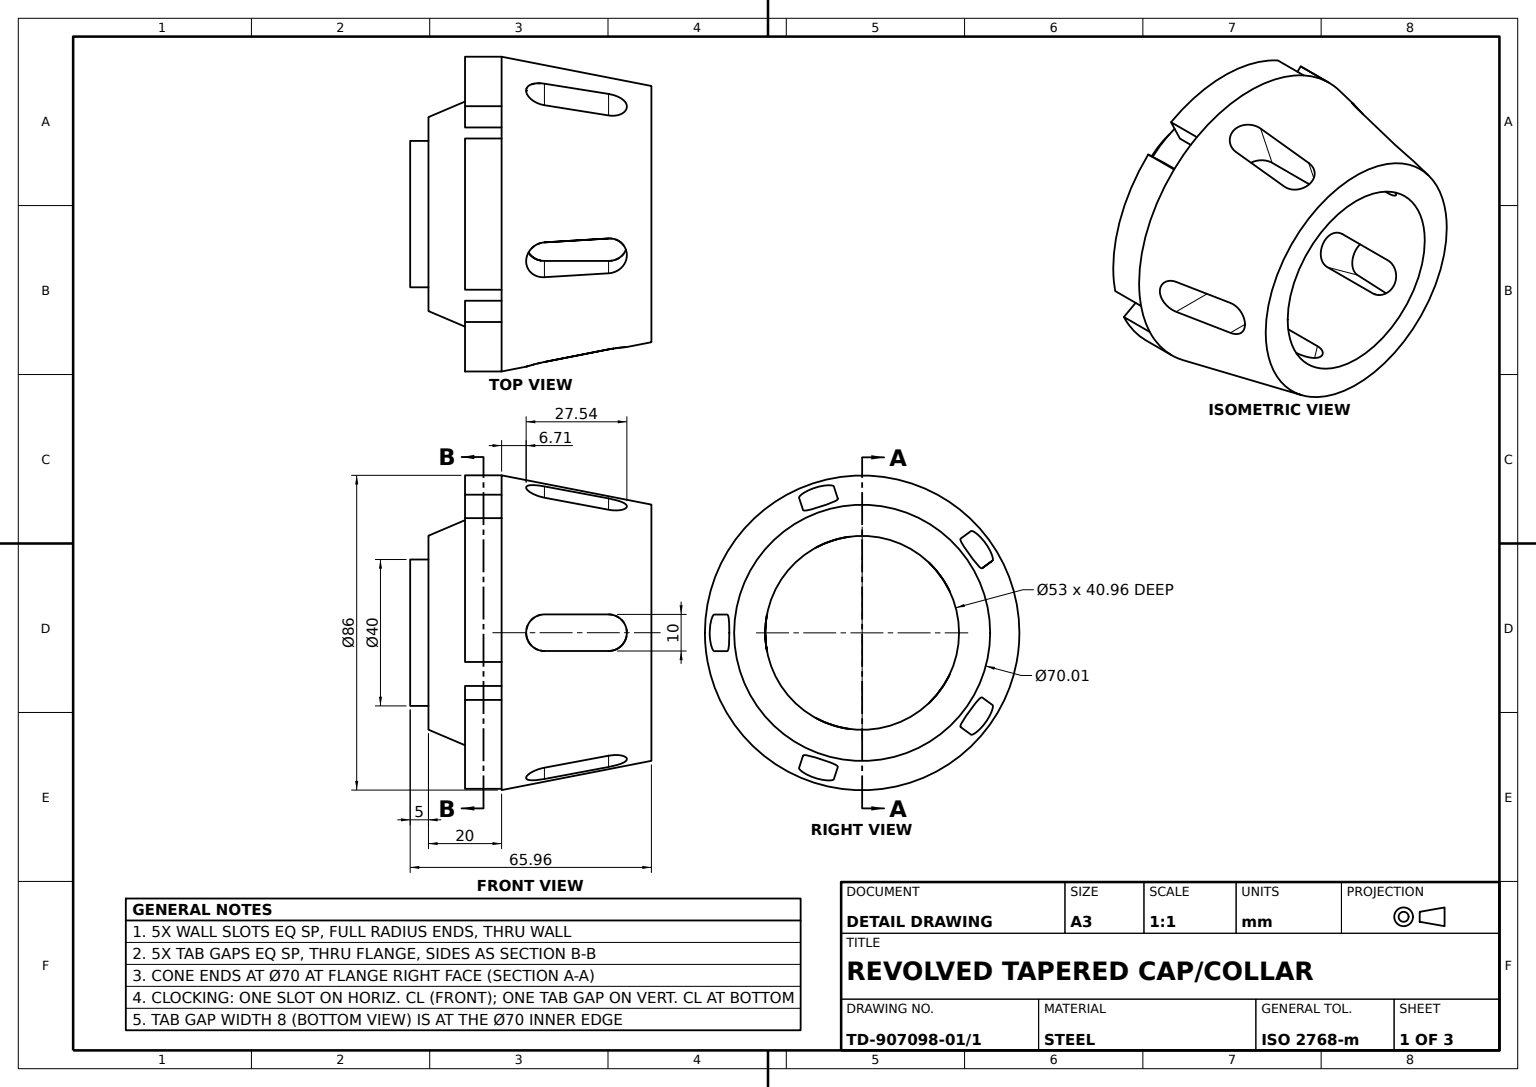
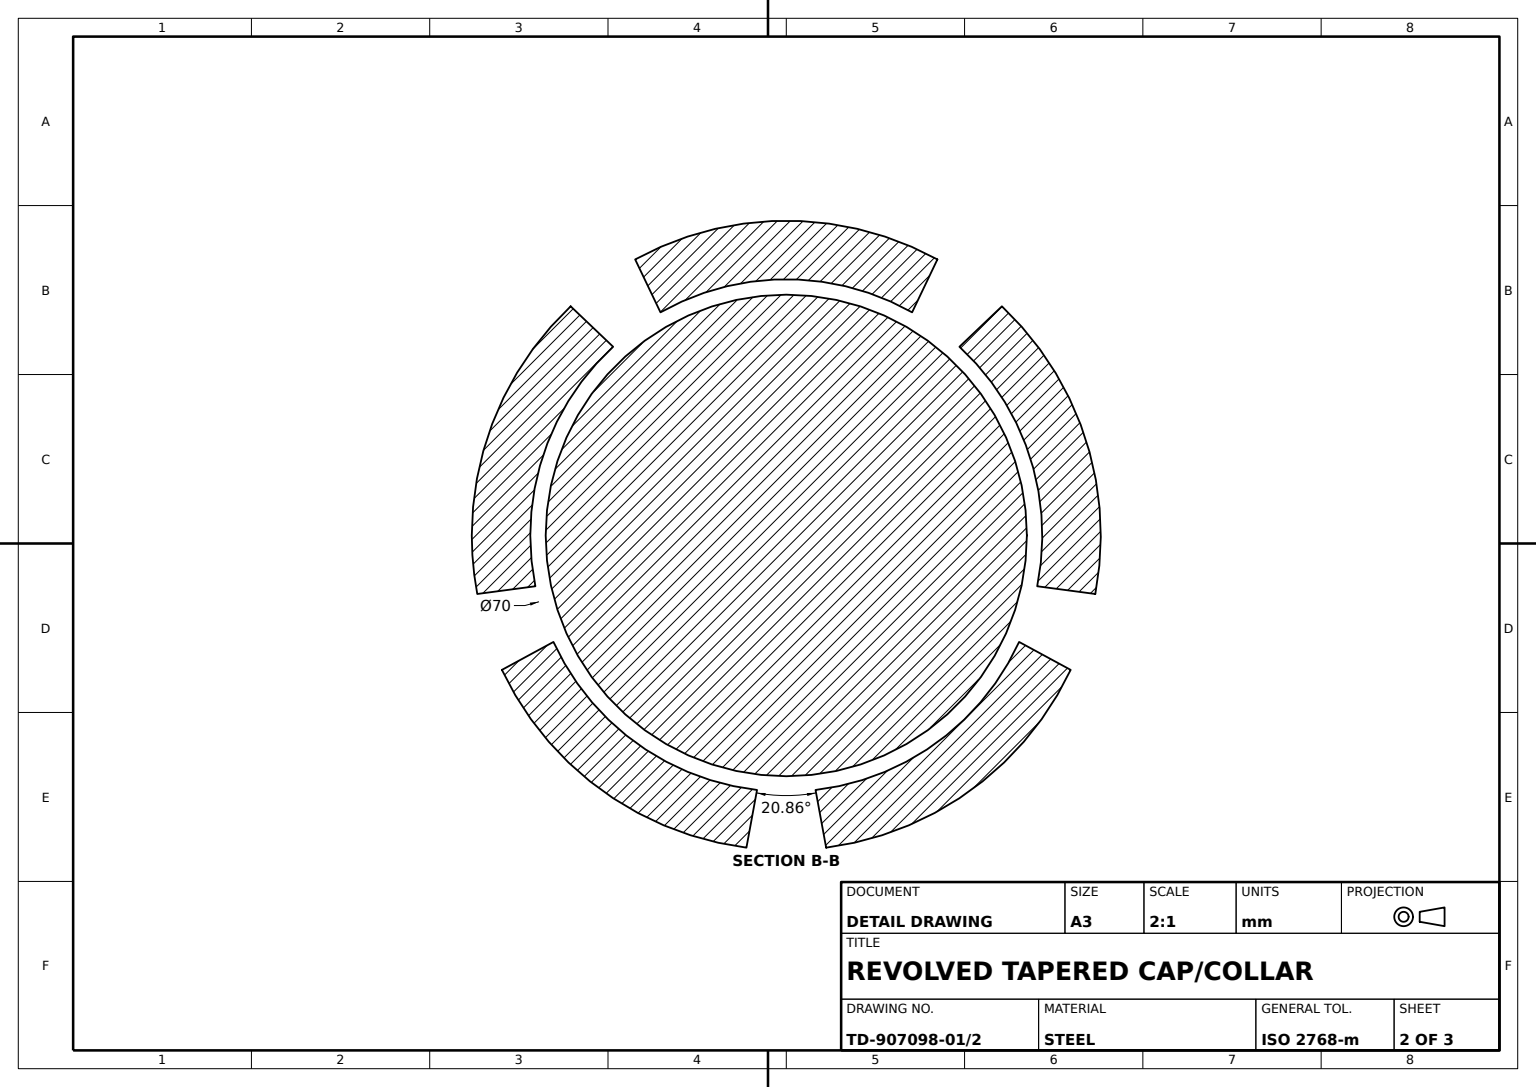
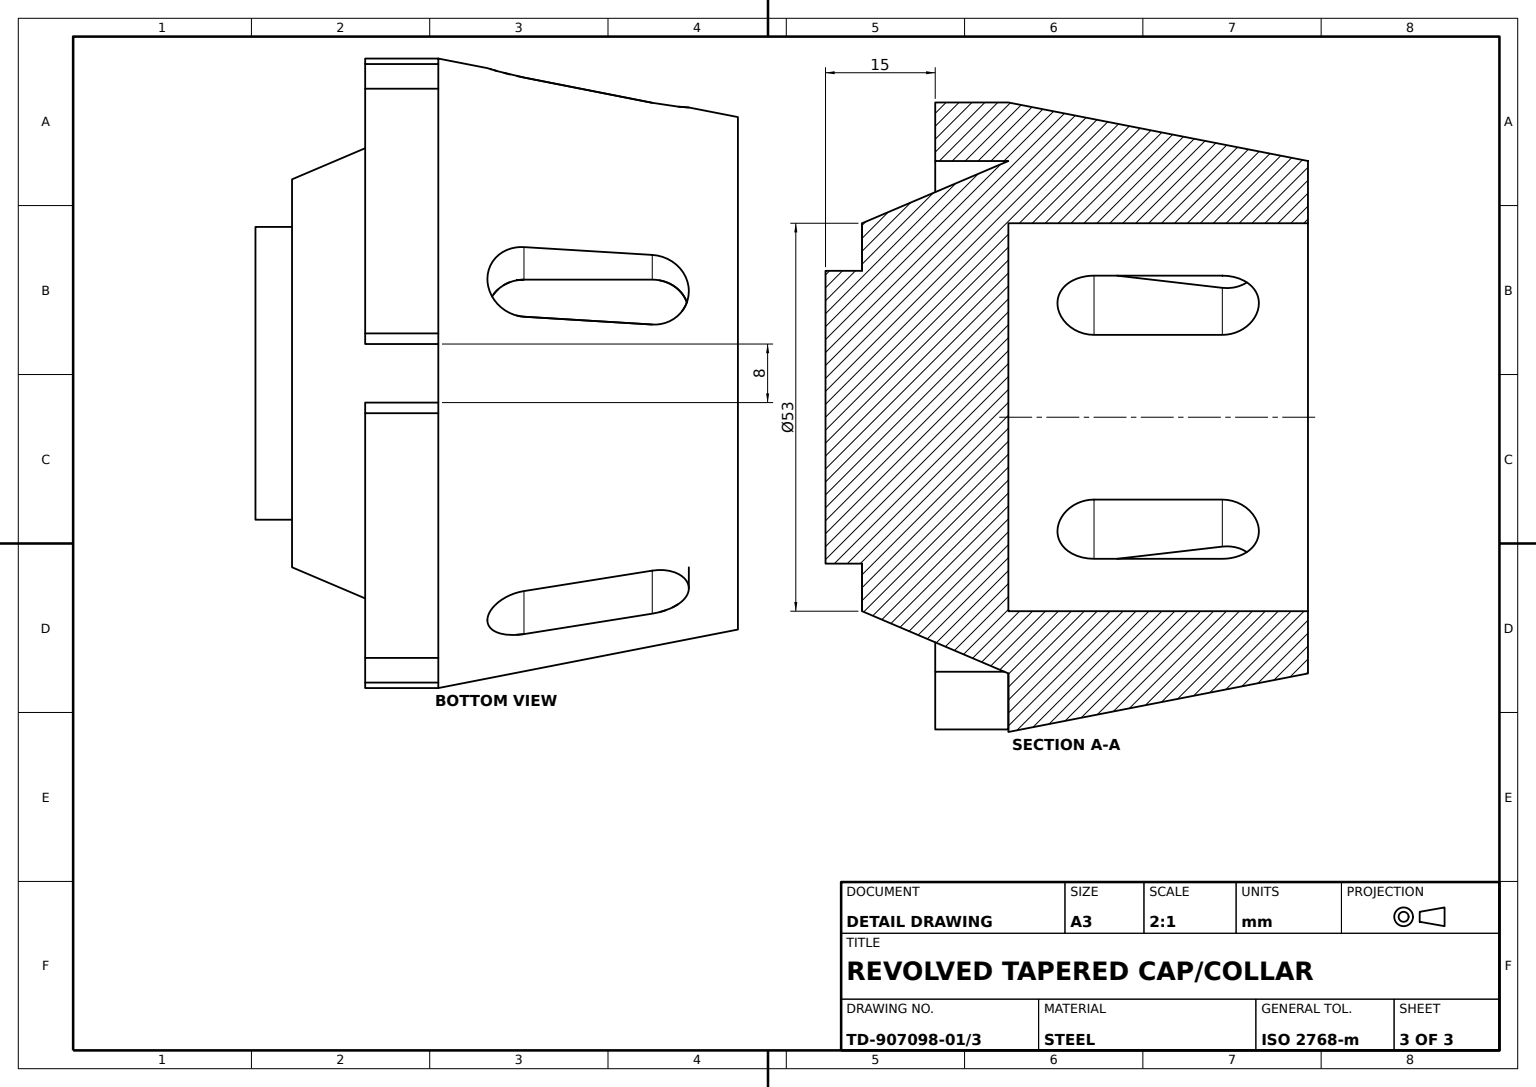
SolidWorks part; units mm, degrees
material "Plain Carbon Steel"
ref_plane "Front Plane" through (0, 0, 0) normal (0, 0, 1) x (1, 0, 0)
ref_plane "Top Plane" through (0, 0, 0) normal (0, 1, 0) x (1, 0, 0)
ref_plane "Right Plane" through (0, 0, 0) normal (1, 0, 0) x (0, 0, -1)
sketch "Housing Profile Sketch" plane through (0, 0, 0) normal (0, 0, 1) x (1, 0, 0)
  line L0 (0, 0) -> (0, 65.96) construction
  line L1 (0, 0) -> (-20, 0)
  line L2 (-20, 0) -> (-20, 5)
  line L3 (-20, 5) -> (-26.5, 5)
  line L4 (-26.5, 5) -> (-35, 25)
  line L5 (-43, 25) -> (-35, 25)
  line L6 (-35.005, 65.96) -> (-26.5, 65.96)
  line L7 (-43, 25) -> (-35.005, 65.96)
  line L9 (0, 0) -> (0, 65.96) construction
  line L10 (-26.5, 65.96) -> (-26.5, 25)
  line L11 (-26.5, 25) -> (0, 25)
  line L12 (0, 25) -> (0, 0)
  dimension "D1" = 20
  dimension "D2" = 5
  dimension "D3" = 70.01
  dimension "D4" = 40
  dimension "D5" = 53
  dimension "D6" = 70
  dimension "D7" = 53
  dimension "D8" = 86
  dimension "D9" = 40.96
revolve "Tapered Housing Body" add sketch "Housing Profile Sketch" angle 360 about L0
sketch "Wall Slot Sketch" plane through (0, 0, 0) normal (0, 0, 1) x (1, 0, 0)
  line L0 (0, 54.25) -> (0, 36.71) construction
  line L1 (5, 54.25) -> (5, 36.71)
  line L2 (-5, 54.25) -> (-5, 36.71)
  line L3 (-43, 25) -> (43, 25) construction
  line L4 (26.5, 65.96) -> (-26.5, 65.96) construction
  arc A0 (5, 54.25) -> (-5, 54.25) centre (0, 54.25) ccw
  arc A1 (-5, 36.71) -> (5, 36.71) centre (0, 36.71) ccw
  point P3 (0, 45.48)
  dimension "D3" = 5
  dimension "D1" = 11.71
  dimension "D2" = 11.71
extrude "Wall Slot Cut" cut sketch "Wall Slot Sketch" along normal up to next
pattern_circular "Wall Slot Pattern 5x" count 5 over 360 about axis through (0, 0, 0) along (0, 1, 0) of "Wall Slot Cut"
sketch "Base Tab Sketch" plane through (0, 25, 0) normal (0, -1, 0) x (1, 0, 0)
  line L2 (0, 0) -> (43, 0) construction
  line L11 (34.7707, 4) -> (42.6531, 5.451)
  line L12 (34.7707, -4) -> (42.6531, -5.451)
  line L13 (14.549, -31.8328) -> (18.3647, -38.8811)
  line L14 (6.9405, -34.3049) -> (7.9964, -42.2499)
  line L15 (-25.7789, -23.6738) -> (-31.3031, -29.4808)
  line L16 (-30.4812, -17.2016) -> (-37.7111, -20.6609)
  line L17 (-30.4812, 17.2016) -> (-37.7111, 20.6609)
  line L18 (-25.7789, 23.6738) -> (-31.3031, 29.4808)
  line L19 (6.9405, 34.3049) -> (7.9964, 42.2499)
  line L20 (14.549, 31.8328) -> (18.3647, 38.8811)
  circle A13 centre (0, 0) radius 43 construction
  circle A15 centre (0, 0) radius 35 construction
  arc A16 (-30.4812, 17.2016) -> (-30.4812, -17.2016) centre (0, 0) ccw
  arc A25 (-37.7111, 20.6609) -> (-37.7111, -20.6609) centre (0, 0) ccw
  arc A26 (6.9405, 34.3049) -> (-25.7789, 23.6738) centre (0, 0) ccw
  arc A27 (14.549, -31.8328) -> (34.7707, -4) centre (0, 0) ccw
  arc A28 (18.3647, -38.8811) -> (42.6531, -5.451) centre (0, 0) ccw
  arc A29 (-25.7789, -23.6738) -> (6.9405, -34.3049) centre (0, 0) ccw
  arc A30 (-31.3031, -29.4808) -> (7.9964, -42.2499) centre (0, 0) ccw
  arc A31 (34.7707, 4) -> (14.549, 31.8328) centre (0, 0) ccw
  arc A32 (42.6531, 5.451) -> (18.3647, 38.8811) centre (0, 0) ccw
  arc A33 (7.9964, 42.2499) -> (-31.3031, 29.4808) centre (0, 0) ccw
  dimension "D2" = 8
  dimension "D1" = 20.86
extrude "Base Tabs" add sketch "Base Tab Sketch" along normal blind 10
